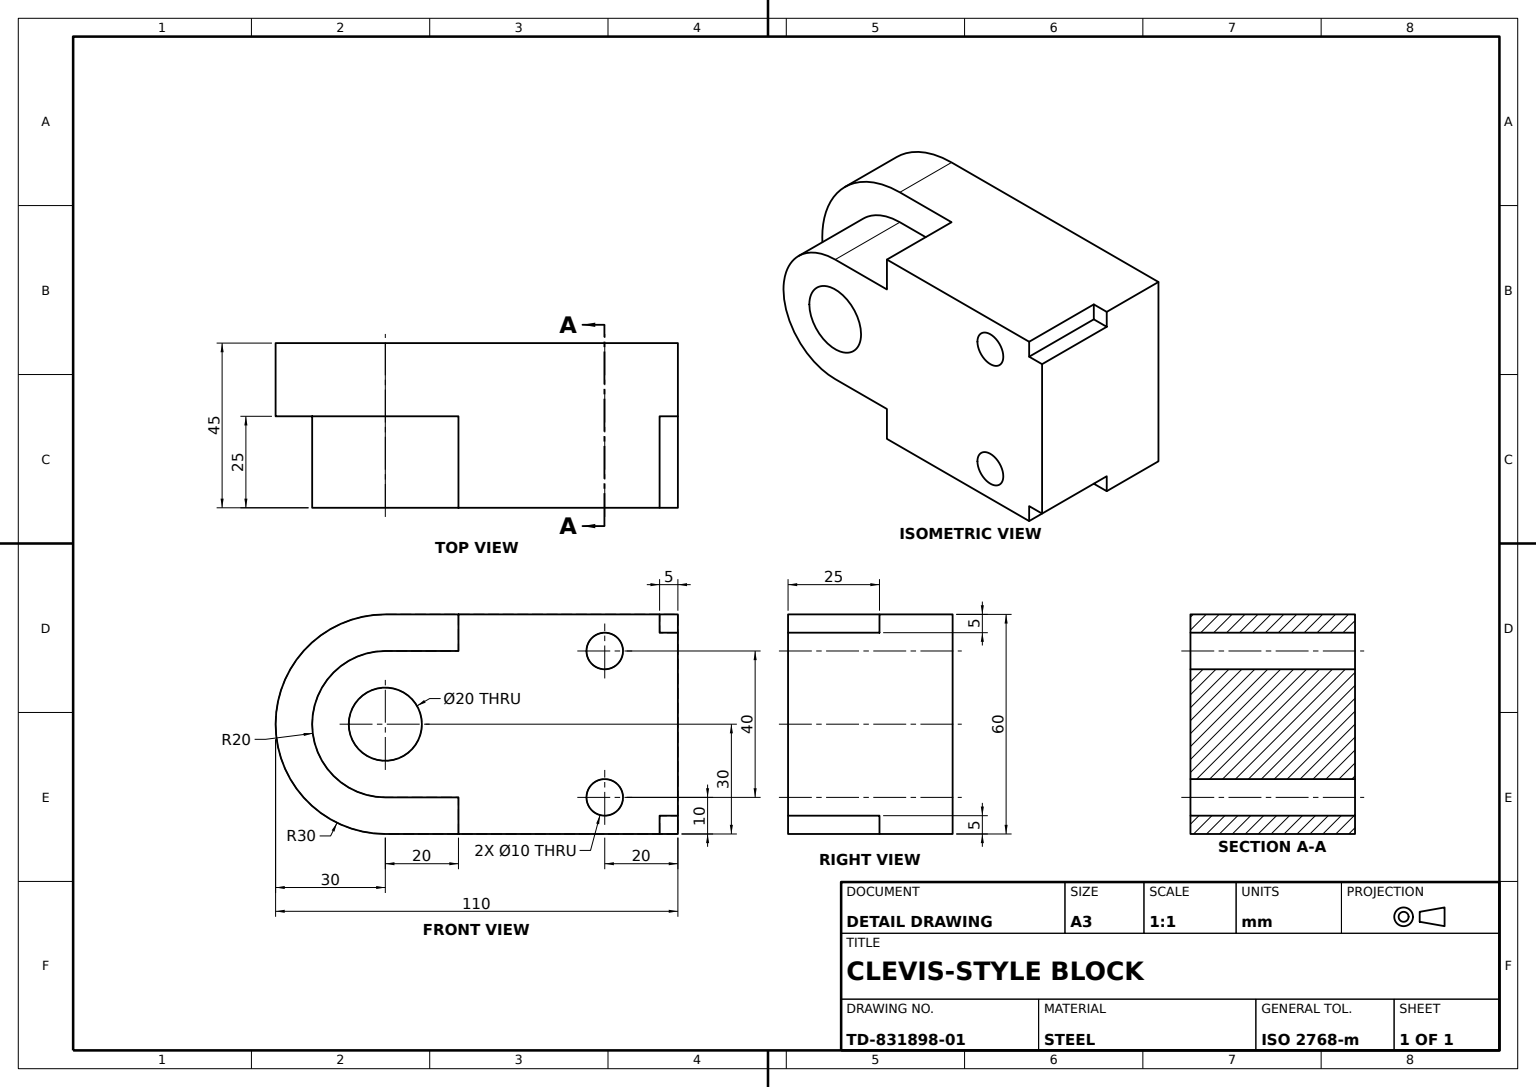
from build123d import *

# Parameters (mm, degrees)
BASE_BLOCK_SKETCH_R       = 10
BASE_BLOCK_DEPTH          = 20
LUG_BOSS_SKETCH_R         = 10
LUG_BOSS_SKETCH_R_2       = 5
LUG_BOSS_WITH_HOLES_DEPTH = 25
SLOT_CUT_SKETCH_R         = 5
SLOT_CUT_DEPTH            = 97.566039579


with BuildPart() as part:
    # Base Block Sketch → Base Block (new body)
    with BuildSketch(Plane.XY):
        with BuildLine():
            Line((0, 30), (80, 30))
            Line((80, 30), (80, -30))
            Line((80, -30), (0, -30))
            ThreePointArc((0, -30), (-30, 0), (0, 30))
        make_face()
        Circle(BASE_BLOCK_SKETCH_R, mode=Mode.SUBTRACT)
    extrude(amount=BASE_BLOCK_DEPTH)

    # Lug Boss Sketch → Lug Boss With Holes (add)
    with BuildSketch(Plane.XY.offset(20)):
        with BuildLine():
            Line((0, 20), (20, 20))
            Line((20, 20), (20, 30))
            Line((20, 30), (75, 30))
            Line((75, 30), (75, 25))
            Line((75, 25), (80, 25))
            Line((80, 25), (80, -25))
            Line((80, -25), (75, -25))
            Line((75, -25), (75, -30))
            Line((75, -30), (20, -30))
            Line((20, -30), (20, -20))
            Line((20, -20), (0, -20))
            ThreePointArc((0, -20), (-20, 0), (0, 20))
        make_face()
        Circle(LUG_BOSS_SKETCH_R, mode=Mode.SUBTRACT)
        with Locations((60, 20)):
            Circle(LUG_BOSS_SKETCH_R_2, mode=Mode.SUBTRACT)
        with Locations((60, -20)):
            Circle(LUG_BOSS_SKETCH_R_2, mode=Mode.SUBTRACT)
    extrude(amount=LUG_BOSS_WITH_HOLES_DEPTH)

    # Slot Cut Sketch → Slot Cut (cut, through all)
    with BuildSketch(Plane.XY.offset(45)):
        with Locations((60, -20)):
            Circle(SLOT_CUT_SKETCH_R)
        with Locations((60, 20)):
            Circle(SLOT_CUT_SKETCH_R)
    extrude(amount=-SLOT_CUT_DEPTH, mode=Mode.SUBTRACT)


solid = part.part
